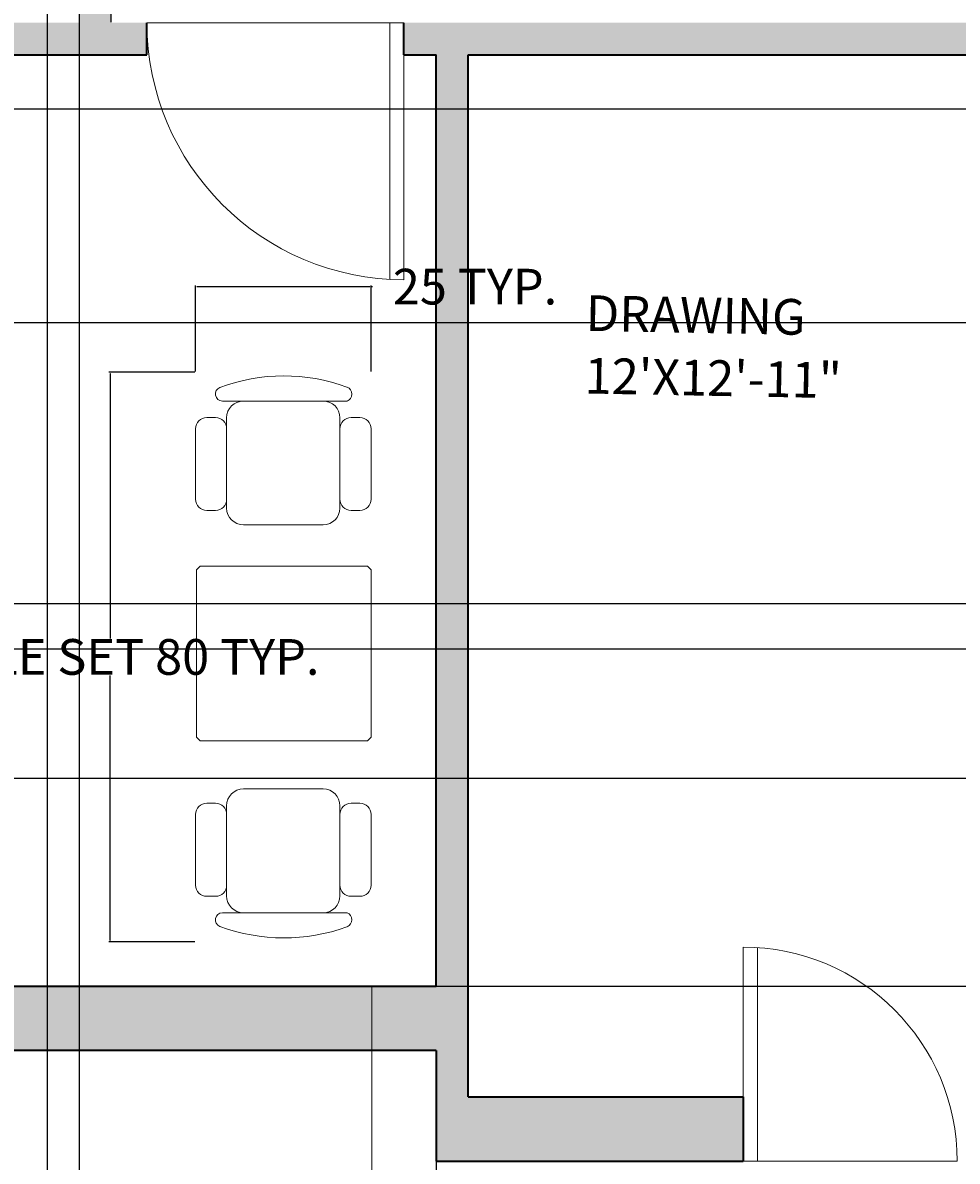
# Model space of a CAD drawing. Units: inches. Extents: x 2807 to 3326, y 2005 to 2580.
# Tile 3 of 12: x 2936 to 3067, y 2120 to 2280. Entities that reach past the tile are written whole.
import ezdxf

# ---------------------------------------------------------------- set-up
doc = ezdxf.new("R2010")
doc.units = ezdxf.units.IN
doc.header["$LTSCALE"] = 0.4
for name, color, linetype, lineweight in [('A-ANNO-DIMS', 2, 'Continuous', 18), ('A-AREA-IDEN', 5, 'Continuous', 18), ('A-FLOR-STRS', 233, 'Continuous', 18), ('A-WALL-PATT', 231, 'Continuous', 13), ('DOORS', 144, 'Continuous', 18), ('Furniture', 7, 'Continuous', 15), ('WALL', 233, 'Continuous', 35)]:
    doc.layers.add(name, color=color, linetype=linetype, lineweight=lineweight)
doc.styles.get("Standard").update_dxf_attribs({"font": 'txt', "height": 5})
doc.dimstyles.get("Standard").update_dxf_attribs({"dimtxt": 0.18, "dimasz": 0.18, "dimexe": 0.18, "dimexo": 0.0625, "dimgap": 0.09, "dimtad": 0, "dimtih": 1, "dimtoh": 1, "dimdec": 4, "dimzin": 0, "dimdsep": 46, "dimtxsty": 'Standard', "dimcen": 0.09, "dimadec": 0, "dimazin": 0, "dimtfac": 1, "dimtdec": 4, "dimtofl": 0, "dimtmove": 0, "dimatfit": 3, "dimfxl": 1, "dimtolj": 1, "dimtzin": 0, "dimarcsym": 0})

# ---------------------------------------------------------------- blocks, each defined once
blk = doc.blocks.new('DOOR-30')
for p, q in [((0, 0), (-30, 0)), ((-2, -29.93), (-2, 0)), ((0, -30), (0, 0))]:
    blk.add_line(p, q)
blk.add_arc((0, 0), 30, 180, 270)
blk = doc.blocks.new('DOOR-36')
for p, q in [((0, 0), (-36, 0)), ((-2, -35.94), (-2, 0)), ((0, -36), (0, 0))]:
    blk.add_line(p, q)
blk.add_arc((0, 0), 36, 180, 270)
blk = doc.blocks.new('TABLE-SET-TWO')
for p, q in [((-7.94, 35.84), (-8.53, 35.84)), ((8.92, 35.84), (-7.94, 35.84)), ((-5.59, 35.84), (5.59, 35.84)), ((-10.73, 33.54), (-9.51, 33.54)), ((9.51, 33.54), (10.73, 33.54)), ((-12.31, 22.08), (-12.31, 31.97)), ((-7.94, 20.85), (-7.94, 33.49)), ((-7.94, 31.97), (-7.94, 22.08)), ((7.94, 33.49), (7.94, 20.85)), ((7.94, 22.08), (7.94, 31.97)), ((12.31, 31.97), (12.31, 22.08)), ((-9.51, 20.51), (-10.73, 20.51)), ((10.73, 20.51), (9.51, 20.51)), ((5.59, 18.5), (-5.59, 18.5)), ((-12.17, 12.19), (-11.66, 12.7)), ((-12.17, -11.26), (-12.17, 12.19)), ((-11.66, 12.7), (11.79, 12.7)), ((11.79, 12.7), (12.3, 12.19)), ((12.3, 12.19), (12.3, -11.26)), ((-11.66, -11.77), (-12.17, -11.26)), ((11.79, -11.77), (-11.66, -11.77)), ((12.3, -11.26), (11.79, -11.77)), ((5.59, -18.5), (-5.59, -18.5)), ((-9.51, -20.51), (-10.73, -20.51)), ((10.73, -20.51), (9.51, -20.51)), ((-12.31, -22.08), (-12.31, -31.97)), ((-7.94, -20.85), (-7.94, -33.49)), ((-7.94, -31.97), (-7.94, -22.08)), ((7.94, -33.49), (7.94, -20.85)), ((7.94, -22.08), (7.94, -31.97)), ((12.31, -31.97), (12.31, -22.08)), ((-10.73, -33.54), (-9.51, -33.54)), ((9.51, -33.54), (10.73, -33.54)), ((-7.94, -35.84), (-8.53, -35.84)), ((8.92, -35.84), (-7.94, -35.84)), ((-5.59, -35.84), (5.59, -35.84))]:
    blk.add_line(p, q)
for centre, radius, start, end in [((0.09, 13.6), 25.77, 69.9544, 110.3611), ((-8.53, 36.83), 0.986, 110.3611, 270), ((8.57, 36.82), 1.04, 290.0456, 69.9544), ((-5.59, 33.49), 2.35, 90, 180), ((5.59, 33.49), 2.35, 0, 90), ((-10.73, 31.97), 1.57, 90, 180), ((-9.51, 31.97), 1.57, 0, 90), ((9.51, 31.97), 1.57, 90, 180), ((10.73, 31.97), 1.57, 0, 90), ((-10.73, 22.08), 1.57, 180, 270), ((-9.51, 22.08), 1.57, 270, 0), ((-5.59, 20.85), 2.35, 180, 270), ((5.59, 20.85), 2.35, 270, 0), ((9.51, 22.08), 1.57, 180, 270), ((10.73, 22.08), 1.57, 270, 0), ((-5.59, -20.85), 2.35, 90, 180), ((5.59, -20.85), 2.35, 0, 90), ((-10.73, -22.08), 1.57, 90, 180), ((-9.51, -22.08), 1.57, 0, 90), ((9.51, -22.08), 1.57, 90, 180), ((10.73, -22.08), 1.57, 0, 90), ((-10.73, -31.97), 1.57, 180, 270), ((-9.51, -31.97), 1.57, 270, 0), ((-5.59, -33.49), 2.35, 180, 270), ((5.59, -33.49), 2.35, 270, 0), ((9.51, -31.97), 1.57, 180, 270), ((10.73, -31.97), 1.57, 270, 0), ((-8.53, -36.83), 0.986, 90, 249.6389), ((8.57, -36.82), 1.04, 290.0456, 69.9544), ((0.09, -13.6), 25.77, 249.6389, 290.0456)]:
    blk.add_arc(centre, radius, start, end)
blk = doc.blocks.new('*D29')
at = {"layer": 'A-ANNO-DIMS', "color": 0, "lineweight": -2, "ltscale": 0.4, "transparency": 16777216}
for p, q in [((2959.79, 2230.64), (2947.71, 2230.64)), ((2947.89, 2230.46), (2947.89, 2193.32)), ((2947.89, 2151.01), (2947.89, 2188.14)), ((2959.79, 2150.83), (2947.71, 2150.83))]:
    blk.add_line(p, q, dxfattribs=at)
at = {"layer": 'A-ANNO-DIMS', "color": 0, "ltscale": 0.4, "transparency": 16777216}
for points in [[(2947.86, 2230.46), (2947.92, 2230.46), (2947.89, 2230.64)], [(2947.86, 2151.01), (2947.92, 2151.01), (2947.89, 2150.83)]]:
    blk.add_solid(points, dxfattribs=at)
at = {"layer": 'Defpoints', "color": 0, "ltscale": 0.4, "transparency": 16777216}
for p in [(2947.89, 2230.64), (2959.86, 2230.64), (2959.86, 2150.83)]:
    blk.add_point(p, dxfattribs=at)
at = {"layer": 'A-ANNO-DIMS', "color": 0, "ltscale": 0.4, "transparency": 16777216, "insert": (2947.89, 2190.73), "char_height": 5, "attachment_point": 5}
blk.add_mtext('\\A1;TABLE SET 80 TYP.', dxfattribs=at)
blk = doc.blocks.new('*D30')
at = {"layer": 'A-ANNO-DIMS', "color": 0, "lineweight": -2, "ltscale": 0.4, "transparency": 16777216}
for p, q in [((2959.86, 2230.7), (2959.86, 2242.79)), ((2960.04, 2242.61), (2984.29, 2242.61)), ((2984.47, 2230.7), (2984.47, 2242.79)), ((2984.47, 2242.61), (2984.65, 2242.61))]:
    blk.add_line(p, q, dxfattribs=at)
at = {"layer": 'A-ANNO-DIMS', "color": 0, "ltscale": 0.4, "transparency": 16777216}
for points in [[(2960.04, 2242.64), (2960.04, 2242.58), (2959.86, 2242.61)], [(2984.29, 2242.64), (2984.29, 2242.58), (2984.47, 2242.61)]]:
    blk.add_solid(points, dxfattribs=at)
at = {"layer": 'Defpoints', "color": 0, "ltscale": 0.4, "transparency": 16777216}
for p in [(2984.47, 2242.61), (2959.86, 2230.64), (2984.47, 2230.64)]:
    blk.add_point(p, dxfattribs=at)
at = {"layer": 'A-ANNO-DIMS', "color": 0, "ltscale": 0.4, "transparency": 16777216, "insert": (2999.02, 2242.61), "char_height": 5, "attachment_point": 5}
blk.add_mtext('\\A1;25 TYP.', dxfattribs=at)
blk = doc.blocks.new('*D31')
at = {"layer": 'A-ANNO-DIMS', "color": 0, "lineweight": -2, "ltscale": 0.4, "transparency": 16777216}
for p, q in [((2844.57, 2135.51), (2844.57, 2008.45)), ((3288.57, 2135.51), (3288.57, 2008.45)), ((2844.75, 2008.63), (3059.93, 2008.63)), ((3288.39, 2008.63), (3073.2, 2008.63))]:
    blk.add_line(p, q, dxfattribs=at)
at = {"layer": 'A-ANNO-DIMS', "color": 0, "ltscale": 0.4, "transparency": 16777216}
for points in [[(2844.75, 2008.66), (2844.75, 2008.6), (2844.57, 2008.63)], [(3288.39, 2008.66), (3288.39, 2008.6), (3288.57, 2008.63)]]:
    blk.add_solid(points, dxfattribs=at)
at = {"layer": 'Defpoints', "color": 0, "ltscale": 0.4, "transparency": 16777216}
for p in [(2844.57, 2135.58), (3288.57, 2135.58), (3288.57, 2008.63)]:
    blk.add_point(p, dxfattribs=at)
at = {"layer": 'A-ANNO-DIMS', "color": 0, "ltscale": 0.4, "transparency": 16777216, "insert": (3066.57, 2008.63), "char_height": 5, "attachment_point": 5}
blk.add_mtext('\\A1;444', dxfattribs=at)
blk = doc.blocks.new('*D33')
at = {"layer": 'A-ANNO-DIMS', "color": 0, "lineweight": -2, "ltscale": 0.4, "transparency": 16777216}
for p, q in [((2844.504691, 2135.576496), (2816.937191, 2135.576496)), ((2817.117191, 2135.396496), (2817.117191, 2088.416496)), ((2817.117191, 2036.256496), (2817.117191, 2083.236496)), ((2984.504691, 2036.076496), (2816.937191, 2036.076496))]:
    blk.add_line(p, q, dxfattribs=at)
at = {"layer": 'A-ANNO-DIMS', "color": 0, "ltscale": 0.4, "transparency": 16777216}
for points in [[(2817.087191, 2135.396496), (2817.147191, 2135.396496), (2817.117191, 2135.576496)], [(2817.087191, 2036.256496), (2817.147191, 2036.256496), (2817.117191, 2036.076496)]]:
    blk.add_solid(points, dxfattribs=at)
at = {"layer": 'Defpoints', "color": 0, "ltscale": 0.4, "transparency": 16777216}
for p in [(2817.117191, 2135.576496), (2844.567191, 2135.576496), (2984.567191, 2036.076496)]:
    blk.add_point(p, dxfattribs=at)
at = {"layer": 'A-ANNO-DIMS', "color": 0, "ltscale": 0.4, "transparency": 16777216, "insert": (2817.117191, 2085.826496), "char_height": 5, "attachment_point": 5}
blk.add_mtext('\\A1;99.5', dxfattribs=at)
blk = doc.blocks.new('*D35')
at = {"layer": 'A-ANNO-DIMS', "color": 0, "lineweight": -2, "ltscale": 0.4, "transparency": 16777216}
for p, q in [((2844.57, 2135.51), (2844.57, 2107.95)), ((2993.57, 2135.51), (2993.57, 2107.95)), ((2844.75, 2108.13), (2913.14, 2108.13)), ((2993.39, 2108.13), (2924.99, 2108.13))]:
    blk.add_line(p, q, dxfattribs=at)
at = {"layer": 'A-ANNO-DIMS', "color": 0, "ltscale": 0.4, "transparency": 16777216}
for points in [[(2844.75, 2108.16), (2844.75, 2108.1), (2844.57, 2108.13)], [(2993.39, 2108.16), (2993.39, 2108.1), (2993.57, 2108.13)]]:
    blk.add_solid(points, dxfattribs=at)
at = {"layer": 'Defpoints', "color": 0, "ltscale": 0.4, "transparency": 16777216}
for p in [(2844.57, 2135.58), (2993.57, 2135.58), (2844.57, 2108.13)]:
    blk.add_point(p, dxfattribs=at)
at = {"layer": 'A-ANNO-DIMS', "color": 0, "ltscale": 0.4, "transparency": 16777216, "insert": (2919.07, 2108.13), "char_height": 5, "attachment_point": 5}
blk.add_mtext('\\A1;149', dxfattribs=at)
blk = doc.blocks.new('*D45')
at = {"layer": 'A-ANNO-DIMS', "color": 0, "lineweight": -2, "ltscale": 0.4, "transparency": 16777216}
for p, q in [((3279.504691, 2191.826496), (2816.937191, 2191.826496)), ((2817.117191, 2191.646496), (2817.117191, 2170.791496)), ((2817.117191, 2144.756496), (2817.117191, 2165.611496)), ((3279.504691, 2144.576496), (2816.937191, 2144.576496))]:
    blk.add_line(p, q, dxfattribs=at)
at = {"layer": 'A-ANNO-DIMS', "color": 0, "ltscale": 0.4, "transparency": 16777216}
for points in [[(2817.087191, 2191.646496), (2817.147191, 2191.646496), (2817.117191, 2191.826496)], [(2817.087191, 2144.756496), (2817.147191, 2144.756496), (2817.117191, 2144.576496)]]:
    blk.add_solid(points, dxfattribs=at)
at = {"layer": 'Defpoints', "color": 0, "ltscale": 0.4, "transparency": 16777216}
for p in [(2817.117191, 2191.826496), (3279.567191, 2191.826496), (3279.567191, 2144.576496)]:
    blk.add_point(p, dxfattribs=at)
at = {"layer": 'A-ANNO-DIMS', "color": 0, "ltscale": 0.4, "transparency": 16777216, "insert": (2817.117191, 2168.201496), "char_height": 5, "attachment_point": 5}
blk.add_mtext('\\A1;47.25', dxfattribs=at)
blk = doc.blocks.new('*D61')
at = {"layer": 'A-ANNO-DIMS', "color": 0, "lineweight": -2, "ltscale": 0.4, "transparency": 16777216}
for p, q in [((3088.922898, 2267.452063), (2816.937191, 2267.452063)), ((2817.117191, 2267.272063), (2817.117191, 2223.175564)), ((2817.117191, 2173.899065), (2817.117191, 2217.995564)), ((3079.479513, 2173.719065), (2816.937191, 2173.719065))]:
    blk.add_line(p, q, dxfattribs=at)
at = {"layer": 'A-ANNO-DIMS', "color": 0, "ltscale": 0.4, "transparency": 16777216}
for points in [[(2817.087191, 2267.272063), (2817.147191, 2267.272063), (2817.117191, 2267.452063)], [(2817.087191, 2173.899065), (2817.147191, 2173.899065), (2817.117191, 2173.719065)]]:
    blk.add_solid(points, dxfattribs=at)
at = {"layer": 'Defpoints', "color": 0, "ltscale": 0.4, "transparency": 16777216}
for p in [(2817.117191, 2267.452063), (3088.985398, 2267.452063), (3079.542013, 2173.719065)]:
    blk.add_point(p, dxfattribs=at)
at = {"layer": 'A-ANNO-DIMS', "color": 0, "ltscale": 0.4, "transparency": 16777216, "insert": (2817.117191, 2220.585564), "char_height": 5, "attachment_point": 5}
blk.add_mtext('\\A1;93.73', dxfattribs=at)
blk = doc.blocks.new('*D65')
at = {"layer": 'A-ANNO-DIMS', "color": 0, "lineweight": -2, "ltscale": 0.4, "transparency": 16777216}
for p, q in [((3080.36, 2237.55), (2816.94, 2237.55)), ((2817.12, 2237.37), (2817.12, 2220.44)), ((2817.12, 2198.33), (2817.12, 2215.26)), ((3080.36, 2198.15), (2816.94, 2198.15))]:
    blk.add_line(p, q, dxfattribs=at)
at = {"layer": 'A-ANNO-DIMS', "color": 0, "ltscale": 0.4, "transparency": 16777216}
for points in [[(2817.09, 2237.37), (2817.15, 2237.37), (2817.12, 2237.55)], [(2817.09, 2198.33), (2817.15, 2198.33), (2817.12, 2198.15)]]:
    blk.add_solid(points, dxfattribs=at)
at = {"layer": 'Defpoints', "color": 0, "ltscale": 0.4, "transparency": 16777216}
for p in [(2817.12, 2237.55), (3080.43, 2237.55), (3080.43, 2198.15)]:
    blk.add_point(p, dxfattribs=at)
at = {"layer": 'A-ANNO-DIMS', "color": 0, "ltscale": 0.4, "transparency": 16777216, "insert": (2817.12, 2217.85), "char_height": 5, "attachment_point": 5}
blk.add_mtext('\\A1;39.4', dxfattribs=at)
blk = doc.blocks.new('*D69')
at = {"layer": 'A-ANNO-DIMS', "color": 0, "lineweight": -2, "ltscale": 0.4, "transparency": 16777216}
for p, q in [((2939.07, 2380.01), (2939.07, 2008.45)), ((2943.57, 2380.01), (2943.57, 2008.45)), ((2939.25, 2008.63), (2943.39, 2008.63)), ((2943.57, 2008.63), (2943.75, 2008.63))]:
    blk.add_line(p, q, dxfattribs=at)
at = {"layer": 'A-ANNO-DIMS', "color": 0, "ltscale": 0.4, "transparency": 16777216}
for points in [[(2939.25, 2008.66), (2939.25, 2008.6), (2939.07, 2008.63)], [(2943.39, 2008.66), (2943.39, 2008.6), (2943.57, 2008.63)]]:
    blk.add_solid(points, dxfattribs=at)
at = {"layer": 'Defpoints', "color": 0, "ltscale": 0.4, "transparency": 16777216}
for p in [(2939.07, 2380.08), (2943.57, 2380.08), (2943.57, 2008.63)]:
    blk.add_point(p, dxfattribs=at)
at = {"layer": 'A-ANNO-DIMS', "color": 0, "ltscale": 0.4, "transparency": 16777216, "insert": (2949.08, 2008.63), "char_height": 5, "attachment_point": 5}
blk.add_mtext('\\A1;4.5', dxfattribs=at)
blk = doc.blocks.new('*D72')
at = {"layer": 'A-ANNO-DIMS', "color": 0, "lineweight": -2, "ltscale": 0.4, "transparency": 16777216}
for p, q in [((2948.07, 2279.64), (2948.07, 2307.21)), ((2948.25, 2307.03), (3060.05, 2307.03)), ((3184.89, 2307.03), (3073.09, 2307.03)), ((3185.07, 2279.64), (3185.07, 2307.21))]:
    blk.add_line(p, q, dxfattribs=at)
at = {"layer": 'A-ANNO-DIMS', "color": 0, "ltscale": 0.4, "transparency": 16777216}
for points in [[(2948.25, 2307.06), (2948.25, 2307), (2948.07, 2307.03)], [(3184.89, 2307.06), (3184.89, 2307), (3185.07, 2307.03)]]:
    blk.add_solid(points, dxfattribs=at)
at = {"layer": 'Defpoints', "color": 0, "ltscale": 0.4, "transparency": 16777216}
for p in [(3185.07, 2307.03), (2948.07, 2279.58), (3185.07, 2279.58)]:
    blk.add_point(p, dxfattribs=at)
at = {"layer": 'A-ANNO-DIMS', "color": 0, "ltscale": 0.4, "transparency": 16777216, "insert": (3066.57, 2307.03), "char_height": 5, "attachment_point": 5}
blk.add_mtext('\\A1;237', dxfattribs=at)

msp = doc.modelspace()

# ---------------------------------------------------------------- hatches: boundary and pattern name
at = {"layer": 'A-WALL-PATT', "ltscale": 0.4}
h = msp.add_hatch(color=256, dxfattribs=at)
h.dxf.hatch_style = 1
h.paths.add_polyline_path([(3288.5672, 2549.5765), (2941.5672, 2549.5765), (2941.5672, 2540.5765), (2993.5672, 2540.5765), (2993.5672, 2489.5693), (2998.0672, 2489.5693), (2998.0672, 2540.5765), (3135.0672, 2540.5765), (3135.0672, 2479.0765), (3139.5672, 2479.0765), (3139.5672, 2540.5765), (3279.5672, 2540.5765), (3279.5672, 2510.5765), (3288.5672, 2510.5765)])
h.paths.add_polyline_path([(2905.5672, 2549.5765), (2844.5672, 2549.5765), (2844.5672, 2445.94), (2853.5672, 2445.94), (2853.5672, 2540.5765), (2905.5672, 2540.5765)])
h.paths.add_polyline_path([(2853.5672, 2409.94), (2844.5672, 2409.94), (2844.5672, 2371.3497), (2853.5672, 2371.3497), (2853.5672, 2380.0765), (2909.0672, 2380.0765), (2909.0672, 2384.5765), (2853.5672, 2384.5765)])
h.paths.add_polyline_path([(2998.0672, 2389.0765), (2993.5672, 2389.0765), (2993.5672, 2384.5765), (2939.0672, 2384.5765), (2939.0672, 2380.0765), (2943.5672, 2380.0765), (2943.5672, 2314.0765), (2948.0672, 2314.0765), (2948.0672, 2380.0765), (2998.0672, 2380.0765)])
h.paths.add_polyline_path([(2998.0672, 2471.8029), (2993.5672, 2471.8029), (2993.5672, 2425.0765), (2998.0672, 2425.0765)])
h.paths.add_polyline_path([(2953.0672, 2279.5765), (2948.0672, 2279.5765), (2948.0672, 2284.0765), (2943.5672, 2284.0765), (2943.5672, 2279.5765), (2853.5672, 2279.5765), (2853.5672, 2289.0663), (2844.5672, 2289.0663), (2844.5672, 2227.8961), (2853.5672, 2227.8961), (2853.5672, 2275.0765), (2953.0672, 2275.0765)])
h.paths.add_polyline_path([(2943.5672, 2332.0765), (2853.5672, 2332.0765), (2853.5672, 2347.3497), (2844.5672, 2347.3497), (2844.5672, 2313.0663), (2853.5672, 2313.0663), (2853.5672, 2327.5765), (2943.5672, 2327.5765)])
h.paths.add_polyline_path([(3144.0672, 2279.5765), (2993.5672, 2279.5765), (2989.0672, 2279.5765), (2989.0672, 2275.0765), (2993.5672, 2275.0765), (2993.5672, 2144.5765), (2984.5672, 2144.5765), (2984.5672, 2135.5765), (2993.5672, 2135.5765), (2993.5672, 2120.0765), (3036.5672, 2120.0765), (3036.5672, 2129.0765), (2998.0672, 2129.0765), (2998.0672, 2275.0765), (3135.0672, 2275.0765), (3135.0672, 2129.0765), (3096.5672, 2129.0765), (3096.5672, 2120.0765), (3139.5672, 2120.0765), (3139.5672, 2135.5765), (3148.5672, 2135.5765), (3148.5672, 2144.5765), (3139.5672, 2144.5765), (3139.5672, 2275.0765), (3144.0672, 2275.0765)])
h.paths.add_polyline_path([(2984.5672, 2144.5765), (2925.9914, 2144.5765), (2925.9914, 2135.5765), (2984.5672, 2135.5765)])
h.paths.add_polyline_path([(2889.9914, 2144.5765), (2853.5672, 2144.5765), (2853.5672, 2191.8961), (2844.5672, 2191.8961), (2844.5672, 2135.5765), (2889.9914, 2135.5765)])
h.paths.add_polyline_path([(3196.0672, 2144.5765), (3148.5672, 2144.5765), (3148.5672, 2135.5765), (3196.0672, 2135.5765)])
h.paths.add_polyline_path([(3288.5672, 2191.8265), (3279.5672, 2191.8265), (3279.5672, 2144.5765), (3232.0672, 2144.5765), (3232.0672, 2135.5765), (3288.5672, 2135.5765)])
h.paths.add_polyline_path([(3288.5672, 2292.8229), (3279.5672, 2292.8229), (3279.5672, 2291.4371), (3279.5672, 2279.5765), (3189.5672, 2279.5765), (3189.5672, 2293.0765), (3185.0672, 2293.0765), (3185.0672, 2279.5765), (3180.0672, 2279.5765), (3180.0672, 2275.0765), (3279.5672, 2275.0765), (3279.5672, 2227.8265), (3288.5672, 2227.8265)])
h.paths.add_polyline_path([(3288.5672, 2368.0765), (3279.5672, 2368.0765), (3279.5672, 2332.0765), (3174.0672, 2332.0765), (3174.0672, 2327.5765), (3185.0672, 2327.5765), (3189.5672, 2327.5765), (3279.5672, 2327.5765), (3279.5672, 2316.8229), (3288.5672, 2316.8229)])
h.paths.add_polyline_path([(3288.5672, 2474.5765), (3279.5672, 2474.5765), (3279.5672, 2444.5765), (3139.5672, 2444.5765), (3139.5672, 2449.0765), (3135.0672, 2449.0765), (3135.0672, 2327.5765), (3144.0672, 2327.5765), (3144.0672, 2332.0765), (3139.5672, 2332.0765), (3139.5672, 2440.0765), (3279.5672, 2440.0765), (3279.5672, 2404.0765), (3288.5672, 2404.0765)])

# ---------------------------------------------------------------- linework, layer by layer
at = {"layer": 'A-FLOR-STRS'}
msp.add_line((2984.5672, 2144.5765), (2984.5672, 2036.0765), dxfattribs=at)
at = {"layer": 'WALL'}
for p, q in [((2953.0672, 2275.0765), (2953.0672, 2279.5765)), ((2989.0672, 2275.0765), (2989.0672, 2279.5765)), ((2853.5672, 2275.0765), (2953.0672, 2275.0765)), ((2989.0672, 2275.0765), (2993.5672, 2275.0765)), ((2993.5672, 2144.5765), (2993.5672, 2275.0765)), ((2998.0672, 2129.0765), (2998.0672, 2275.0765)), ((2998.0672, 2275.0765), (3135.0672, 2275.0765)), ((2993.5672, 2144.5765), (2853.5672, 2144.5765)), ((2993.5672, 2135.5765), (2844.5672, 2135.5765)), ((2993.5672, 2135.5765), (2993.5672, 2120.0765)), ((2998.0672, 2129.0765), (3036.5672, 2129.0765)), ((3036.5672, 2129.0765), (3036.5672, 2120.0765)), ((2993.5672, 2120.0765), (3036.5672, 2120.0765))]:
    msp.add_line(p, q, dxfattribs=at)

# ---------------------------------------------------------------- block references
at = {"layer": 'DOORS'}
msp.add_blockref('DOOR-36', (2989.0672, 2279.5765), dxfattribs=at)
at = {"layer": 'DOORS', "rotation": 180}
msp.add_blockref('DOOR-30', (3036.5672, 2120.0765), dxfattribs=at)
at = {"layer": 'Furniture'}
msp.add_blockref('TABLE-SET-TWO', (2972.1625, 2190.734), dxfattribs=at)

# ---------------------------------------------------------------- texts
at = {"layer": 'A-AREA-IDEN', "ltscale": 0.4}
for s, p in [('DRAWING ', (3014.4908, 2236.4152)), ('12\'X12\'-11"', (3014.3275, 2227.6428))]:
    msp.add_text(s, height=5, rotation=358.933415, dxfattribs=at).set_placement(p)

# ---------------------------------------------------------------- dimensions: what is measured, and where the dimension line sits
at = {"layer": 'A-ANNO-DIMS', "ltscale": 0.4}
for base, p1, p2, override, picture, middle in [((2943.5672, 2008.6265), (2939.0672, 2380.0765), (2943.5672, 2380.0765), {"dimdec": 1, "dimlfac": 1, "dimrnd": 0, "dimzin": 0, "dimdsep": 46, "dimlunit": 2}, '*D69', (2949.0753, 2008.6265)), ((3288.5672, 2008.6265), (2844.5672, 2135.5765), (3288.5672, 2135.5765), {"dimdec": 0, "dimlfac": 1, "dimrnd": 0, "dimzin": 0, "dimdsep": 46, "dimlunit": 2}, '*D31', (3066.5672, 2008.6265))]:
    dim = msp.add_linear_dim(base=base, p1=p1, p2=p2, dimstyle='Standard', override=override, dxfattribs=at)
    dim.commit()
    dim.dimension.update_dxf_attribs({"geometry": picture, "text_midpoint": middle})
for base, p1, p2, angle, override, picture, middle in [((3185.0672, 2307.0265), (2948.0672, 2279.5765), (3185.0672, 2279.5765), 0, {"dimdec": 0, "dimlfac": 1, "dimrnd": 0, "dimzin": 0, "dimdsep": 46, "dimlunit": 2}, '*D72', (3066.5672, 2307.0265)), ((2817.1172, 2267.4521), (3079.542, 2173.7191), (3088.9854, 2267.4521), 90, {"dimdec": 2, "dimlfac": 1, "dimrnd": 0, "dimzin": 0, "dimdsep": 46, "dimlunit": 2}, '*D61', (2817.1172, 2220.5856)), ((2817.1172, 2237.5518), (3080.4262, 2198.1526), (3080.4262, 2237.5518), 90, {"dimdec": 1, "dimlfac": 1, "dimrnd": 0, "dimzin": 0, "dimdsep": 46, "dimlunit": 2}, '*D65', (2817.1172, 2217.8522)), ((2817.1172, 2191.8265), (3279.5672, 2144.5765), (3279.5672, 2191.8265), 90, {"dimdec": 2, "dimlfac": 1, "dimrnd": 0, "dimzin": 0, "dimdsep": 46, "dimlunit": 2}, '*D45', (2817.1172, 2168.2015)), ((2817.1172, 2135.5765), (2984.5672, 2036.0765), (2844.5672, 2135.5765), 90, {"dimdec": 1, "dimlfac": 1, "dimrnd": 0, "dimzin": 0, "dimdsep": 46, "dimlunit": 2}, '*D33', (2817.1172, 2085.8265)), ((2844.5672, 2108.1265), (2993.5672, 2135.5765), (2844.5672, 2135.5765), 180, {"dimdec": 0, "dimlfac": 1, "dimrnd": 0, "dimzin": 0, "dimdsep": 46, "dimlunit": 2}, '*D35', (2919.0672, 2108.1265))]:
    dim = msp.add_linear_dim(base=base, p1=p1, p2=p2, angle=angle, dimstyle='Standard', override=override, dxfattribs=at)
    dim.commit()
    dim.dimension.update_dxf_attribs({"geometry": picture, "text_midpoint": middle})
dim = msp.add_linear_dim(base=(2984.468, 2242.6069), p1=(2959.8575, 2230.6362), p2=(2984.468, 2230.6362), text='<> TYP.', dimstyle='Standard', override={"dimdec": 0, "dimlfac": 1, "dimrnd": 0, "dimzin": 0, "dimdsep": 46, "dimlunit": 2}, dxfattribs=at)
dim.commit()
dim.dimension.update_dxf_attribs({"geometry": '*D30', "text_midpoint": (2999.0237, 2242.6069)})
dim = msp.add_linear_dim(base=(2947.8868, 2230.6362), p1=(2959.8575, 2150.8316), p2=(2959.8575, 2230.6362), angle=90, text='TABLE SET <> TYP.', dimstyle='Standard', override={"dimdec": 0, "dimlfac": 1, "dimrnd": 0, "dimzin": 0, "dimdsep": 46, "dimlunit": 2}, dxfattribs=at)
dim.commit()
dim.dimension.update_dxf_attribs({"geometry": '*D29', "text_midpoint": (2947.8868, 2190.7339)})

doc.saveas('drawing.dxf')
